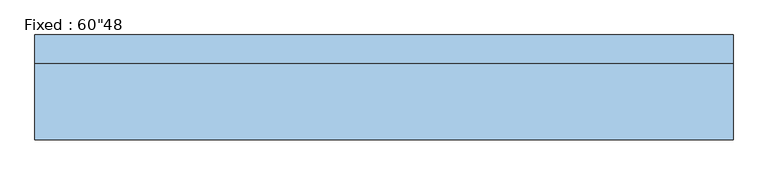
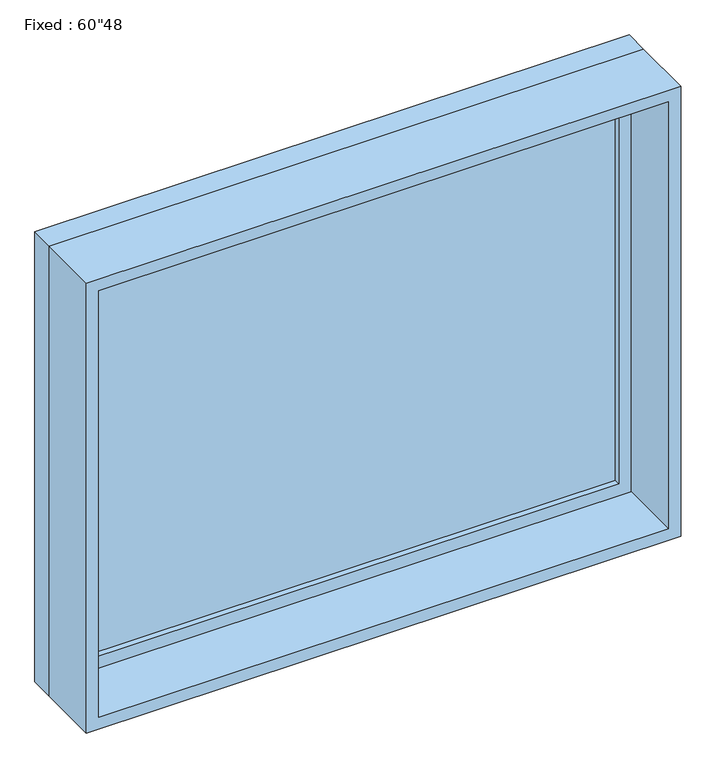
"""IFC4 building model written with IfcOpenShell, lengths in millimetres: window geometry."""

from ifc_helpers import new_model, si_unit, frame, origin, place, context, project, spatial, polyline, outline, extrude, source, transform, mapped, element, save


def window_145d3b12(model_context):
    return source(origin(), model_context, "Body", "SweptSolid", [
        extrude(outline(polyline([(660.4, 66.675), (-736.6, 66.675), (-736.6, 79.375), (660.4, 79.375), (660.4, 66.675)])), frame((0.0, 0.0, 977.9), z_axis=(0.0, 0.0, 1.0), x_axis=(1.0, 0.0, 0.0)), (0.0, 0.0, 1.0), 1092.2),
        extrude(outline(polyline([(2114.55, -781.05), (933.45, -781.05), (933.45, 704.85), (2114.55, 704.85), (2114.55, -781.05)]), holes=[polyline([(2070.1, -736.6), (2070.1, 660.4), (977.9, 660.4), (977.9, -736.6), (2070.1, -736.6)])]), frame((0.0, 50.8, 0.0), z_axis=(0.0, 1.0, 0.0), x_axis=(0.0, 0.0, 1.0)), (0.0, 0.0, 1.0), 44.45),
        extrude(outline(polyline([(2133.6, -800.1), (914.4, -800.1), (914.4, 723.9), (2133.6, 723.9), (2133.6, -800.1)]), holes=[polyline([(2101.85, -768.35), (2101.85, 692.15), (946.15, 692.15), (946.15, -768.35), (2101.85, -768.35)])]), frame((0.0, -114.3, 0.0), z_axis=(0.0, 1.0, 0.0), x_axis=(0.0, 0.0, 1.0)), (0.0, 0.0, 1.0), 165.1),
        extrude(outline(polyline([(2133.6, 723.9), (2133.6, -800.1), (914.4, -800.1), (914.4, 723.9), (2133.6, 723.9)]), holes=[polyline([(2114.55, 704.85), (933.45, 704.85), (933.45, -781.05), (2114.55, -781.05), (2114.55, 704.85)])]), frame((0.0, 50.8, 0.0), z_axis=(0.0, 1.0, 0.0), x_axis=(0.0, 0.0, 1.0)), (0.0, 0.0, 1.0), 63.5),
    ])


if __name__ == "__main__":
    model = new_model("IFC4")
    model_context = context("Model", 3, world=origin())
    ifc_project = project(units=[si_unit("LENGTHUNIT", "METRE", prefix="MILLI")], contexts=[model_context])
    site = spatial("IfcSite", under=ifc_project)
    building = spatial("IfcBuilding", under=site)
    placement = place(None, origin())
    window_shape = window_145d3b12(model_context)
    element("IfcWindow", 1, ObjectType="Fixed : 60\"48", at=placement, inside=building, context=model_context, shape_type="MappedRepresentation", body=[
        mapped(window_shape, transform((0.0, 0.0, 0.0), x_axis=(1.0, 0.0, 0.0), y_axis=(0.0, 1.0, 0.0), z_axis=(0.0, 0.0, 1.0))),
    ])
    save(model, "model.ifc")

# Revit data of these elements
# Type "Fixed : 60\"48"
#   Type Mark = "18"
#   Construction Type Id = "GSP4R"
#   Assembly Code = "B2020100"
#   Analytic Construction = "1/8 in Pilkington single glazing"
#   Visual Light Transmittance = 0.9
#   Solar Heat Gain Coefficient = 0.78
#   Heat Transfer Coefficient (U) = 0.6496 BTU/(h·ft²·°F)
#   Height = 4' - 0"
#   Default Sill Height = 3' - 0"
#   Width = 5' - 0"
#   Window Inset = 0' - 0 3/4"
#   Define Thermal Properties by = 1
#   Glass Pane Material = Glass
#   Sash Material = Sash
#   Wall Closure = (empty or 0)
# Element 1 (IfcWindow, "Fixed : 60\"48")
#   Materials on its faces: "Sash", "Glass"
# Materials
#   "Glass": class "Glass", colour RGB 0 128 192, transparency 0.75, Description = "Soda Lime Glass", Cost = 0
#   "Sash": class "Wood", colour RGB 224 178 126, transparency 0, Cost = 0
